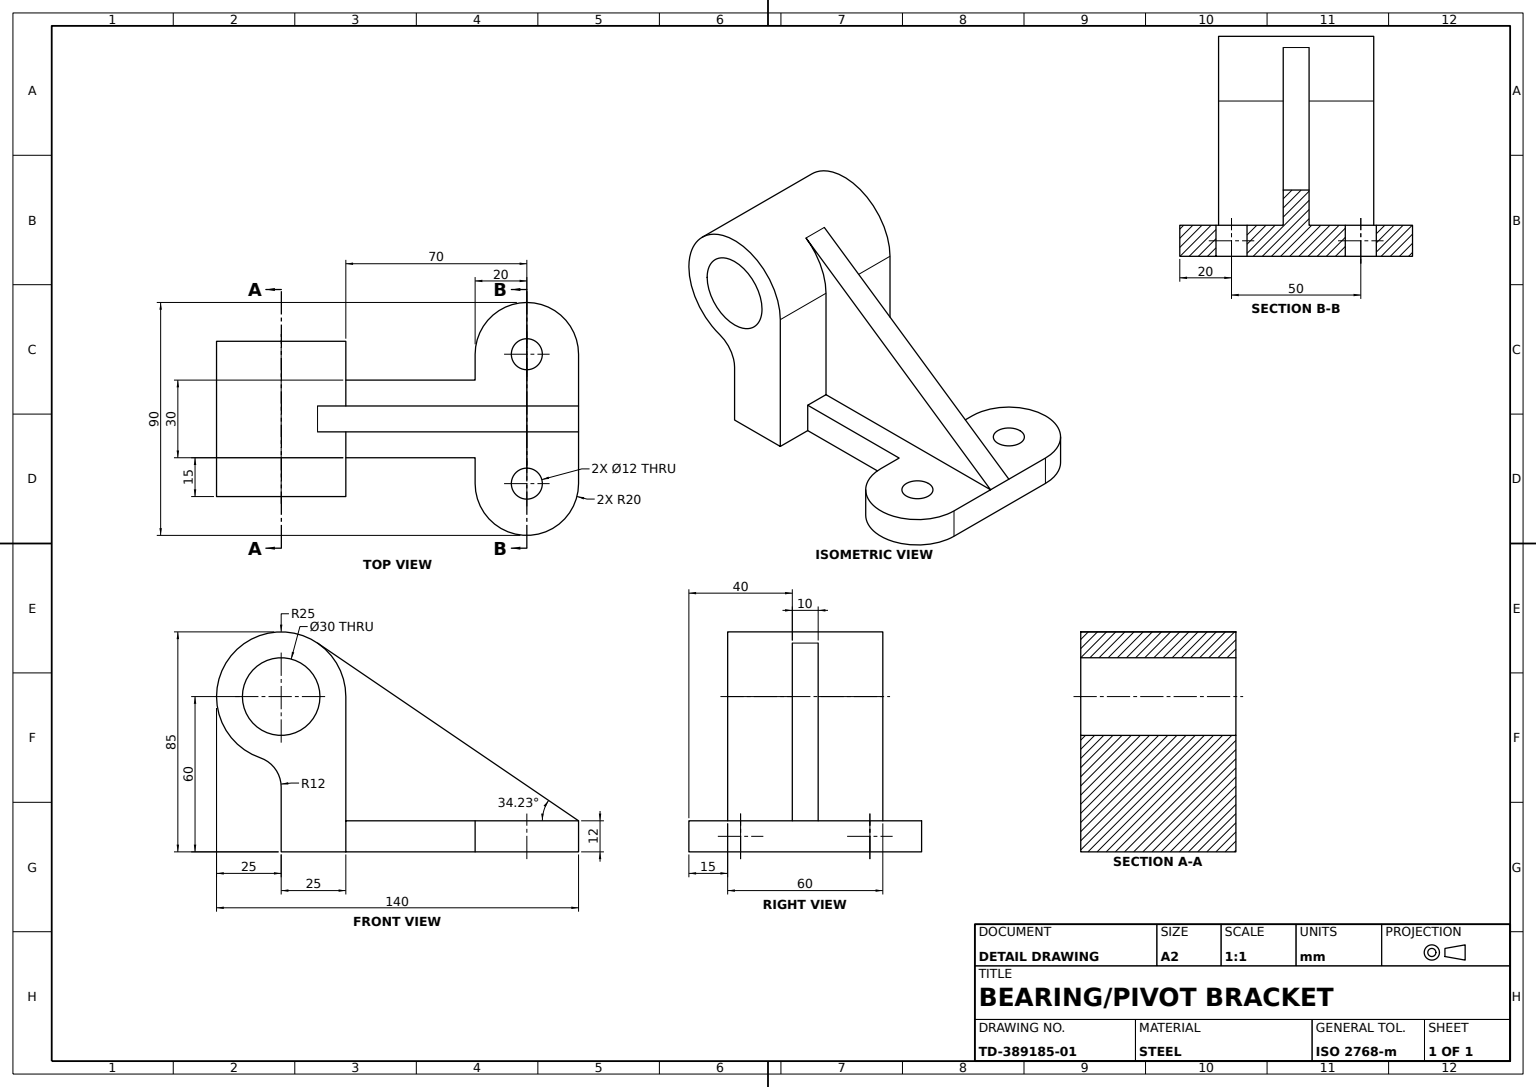
SolidWorks part; units mm, degrees
material "Plain Carbon Steel"
ref_plane "Front Plane" through (0, 0, 0) normal (0, 0, 1) x (1, 0, 0)
ref_plane "Top Plane" through (0, 0, 0) normal (0, 1, 0) x (1, 0, 0)
ref_plane "Right Plane" through (0, 0, 0) normal (1, 0, 0) x (0, 0, -1)
sketch "Base Plate Sketch" plane through (0, 0, 0) normal (0, 1, 0) x (1, 0, 0)
  line L0 (-70, 0) -> (85.3365, 0) construction
  line L1 (0, 25) -> (0, -25) construction
  line L2 (20, 25) -> (20, -25)
  line L3 (-70, -15) -> (-20, -15)
  line L4 (-70, 15) -> (-20, 15)
  line L5 (-20, 25) -> (-20, 15)
  line L6 (-70, -15) -> (85.3365, -15) construction
  line L7 (-70, 15) -> (85.3365, 15) construction
  line L8 (-20, -15) -> (-20, -25)
  line L9 (-70, 15) -> (-70, -15)
  circle A0 centre (0, 25) radius 6
  circle A1 centre (0, -25) radius 6
  arc A2 (20, 25) -> (-20, 25) centre (0, 25) ccw
  arc A3 (-20, -25) -> (20, -25) centre (0, -25) ccw
  dimension "D1" = 50
  dimension "D3" = 12
  dimension "D4" = 40
  dimension "D5" = 30
  dimension "D2" = 70
  dimension "D6" = 15
extrude "Base Plate" add sketch "Base Plate Sketch" along normal mid plane 12
cosmetic thread "Cosmetic Thread1" parameters "D2"=14
cosmetic thread "Cosmetic Thread2" parameters "D2"=14
sketch "Bearing Upright Sketch" plane through (0, 0, 0) normal (0, 0, 1) x (1, 0, 0)
  line L0 (-70, -6) -> (-95, -6)
  line L1 (-95, -6) -> (-95, 19)
  line L2 (-70, -6) -> (-70, 54)
  circle A0 centre (-95, 54) radius 15
  arc A1 (-70, 54) -> (-103.1081, 30.3514) centre (-95, 54) ccw
  arc A2 (-95, 19) -> (-103.1081, 30.3514) centre (-107, 19) ccw
  dimension "D3" = 30
  dimension "D4" = 50
  dimension "D5" = 24
  dimension "D1" = 25
  dimension "D2" = 60
extrude "Bearing Upright" add sketch "Bearing Upright Sketch" along normal mid plane 60
cosmetic thread "Cosmetic Thread3" parameters "D2"=33
sketch "Support Rib Sketch" plane through (0, 0, 0) normal (0, 0, 1) x (1, 0, 0)
  line L0 (20, 6) -> (-80.9377, 74.6701)
  arc A0 (-70, 54) -> (-103.1081, 30.3514) centre (-95, 54) ccw construction
rib "Support Rib 10mm" sketch "Support Rib Sketch" sketch "Support Rib Sketch" thickness 10 extrusion direction parallel to sketch draft on no parameters "D1"=10
